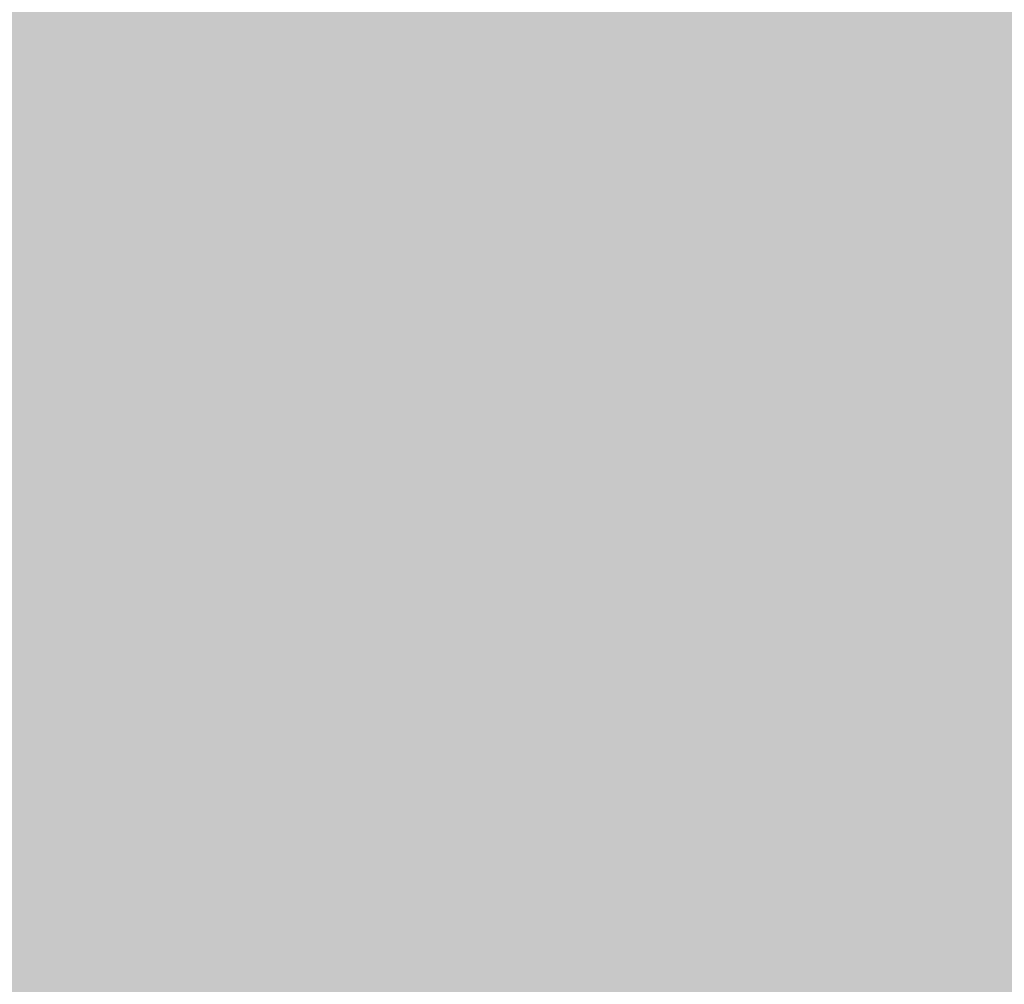
# Model space of a CAD drawing. Units: feet. Extents: x 3168 to 4724, y 827 to 1477.
# Tile 16 of 256: x 3257.5 to 3270.27, y 1074.89 to 1087.4. Entities that reach past the tile are written whole.
import ezdxf

# ---------------------------------------------------------------- set-up
doc = ezdxf.new("R2010")
doc.units = ezdxf.units.FT
doc.layers.add('A-ELEV-PATT', color=8, linetype='Continuous', lineweight=13)

msp = doc.modelspace()

# ---------------------------------------------------------------- hatches: boundary and pattern name
at = {"layer": 'A-ELEV-PATT'}
h = msp.add_hatch(color=256, dxfattribs=at)
h.dxf.hatch_style = 1
edge = h.paths.add_edge_path()
edge.add_ellipse((3552.906, 979.22), major_axis=(36.745, 0), ratio=0.484848, start_angle=0, end_angle=360)
edge = h.paths.add_edge_path()
edge.add_ellipse((3559.892, 929.252), major_axis=(36.745, 0), ratio=0.484848, start_angle=0, end_angle=360)
edge = h.paths.add_edge_path()
edge.add_line((3299.317, 1198.606), (3479.917, 1198.606))
edge.add_line((3479.917, 1198.606), (3479.917, 1209.869))
edge.add_spline(control_points=[(3479.917, 1209.869), (3464.301, 1209.869), (3448.686, 1209.869), (3410.949, 1209.869), (3388.828, 1209.869), (3355.647, 1209.869), (3344.586, 1209.869), (3327.996, 1209.869), (3322.466, 1209.869), (3314.17, 1209.869), (3311.405, 1209.869), (3307.257, 1209.869), (3305.875, 1209.869), (3303.801, 1209.869), (3303.11, 1209.869), (3302.073, 1209.869), (3301.727, 1209.869), (3301.209, 1209.869), (3301.036, 1209.869), (3300.777, 1209.869), (3300.69, 1209.869), (3300.561, 1209.869), (3300.517, 1209.869), (3300.453, 1209.869), (3300.431, 1209.869), (3300.399, 1209.869), (3300.388, 1209.869), (3300.366, 1209.869), (3300.346, 1209.869), (3300.346, 1209.869), (3300.346, 1209.869), (3300.343, 1209.869), (3300.341, 1209.869), (3300.338, 1209.869), (3300.337, 1209.869), (3300.334, 1209.869), (3300.332, 1209.869), (3300.326, 1209.869), (3300.321, 1209.869), (3300.311, 1209.869), (3300.306, 1209.869), (3300.291, 1209.869), (3300.28, 1209.869), (3300.232, 1209.869), (3300.195, 1209.869), (3299.951, 1209.871), (3299.745, 1209.874), (3299.437, 1209.883), (3299.334, 1209.887), (3299.181, 1209.893), (3299.13, 1209.895), (3298.652, 1209.917), (3298.229, 1209.946), (3297.602, 1210.002), (3297.393, 1210.023), (3297.083, 1210.058), (3296.979, 1210.07), (3296.293, 1210.155), (3295.718, 1210.243), (3294.869, 1210.399), (3294.588, 1210.454), (3294.169, 1210.543), (3294.03, 1210.574), (3291.707, 1211.101), (3289.654, 1211.813), (3285.776, 1213.564), (3283.951, 1214.603), (3280.512, 1216.98), (3278.897, 1218.318), (3276.38, 1220.829), (3275.416, 1221.918), (3274.039, 1223.708), (3273.581, 1224.35), (3273.143, 1225.016)], knot_values=[39.119033, 39.119033, 39.119033, 39.119033, 39.286353, 39.286353, 39.523379, 39.523379, 39.641892, 39.641892, 39.701148, 39.701148, 39.730777, 39.730777, 39.745591, 39.745591, 39.752998, 39.752998, 39.756701, 39.756701, 39.758553, 39.758553, 39.759479, 39.759479, 39.759942, 39.759942, 39.760173, 39.760173, 39.760289, 39.760289, 39.760405, 39.760405, 39.760463, 39.760463, 39.763389, 39.763389, 39.764851, 39.764851, 39.767304, 39.767304, 39.773825, 39.773825, 39.78057, 39.78057, 39.79477, 39.79477, 39.845194, 39.845194, 40.126715, 40.126715, 40.267476, 40.267476, 40.337856, 40.337856, 40.927023, 40.927023, 41.221606, 41.221606, 41.368898, 41.368898, 42.202622, 42.202622, 42.619485, 42.619485, 42.827916, 42.827916, 46.118323, 46.118323, 49.408731, 49.408731, 52.699139, 52.699139, 54.927489, 54.927489, 56.104228, 56.104228, 56.104228, 56.104228], weights=[1, 1, 1, 1, 1, 1, 1, 1, 1, 1, 1, 1, 1, 1, 1, 1, 1, 1, 1, 1, 1, 1, 1, 1, 1, 1, 1, 1, 1, 1, 1, 1, 1, 1, 1, 1, 1, 1, 1, 1, 1, 1, 1, 1, 1, 1, 1, 1, 1, 1, 1, 1, 1, 1, 1, 1, 1, 1, 1, 1, 1, 1, 1, 1, 1, 1, 1, 1, 1, 1, 1, 1, 1, 1], degree=3, periodic=0)
edge.add_line((3273.143, 1225.016), (3273.143, 1099.016))
edge.add_line((3273.143, 1099.016), (3299.317, 1099.016))
edge.add_line((3299.317, 1099.016), (3299.317, 1198.606))
edge = h.paths.add_edge_path()
edge.add_line((3304.758, 1324.158), (3479.917, 1324.158))
edge.add_line((3479.917, 1324.158), (3479.917, 1335.715))
edge.add_line((3479.917, 1335.715), (3269.162, 1335.715))
edge.add_spline(control_points=[(3269.162, 1335.715), (3264.024, 1335.715), (3258.364, 1328.958), (3259.264, 1323.9)], knot_values=[0, 0, 0, 0, 15.412191, 15.412191, 15.412191, 15.412191], degree=3, periodic=0)
edge.add_line((3259.264, 1323.9), (3265.517, 1288.769))
edge.add_line((3265.517, 1288.769), (3275.265, 1261.546))
edge.add_line((3275.265, 1261.546), (3304.758, 1261.546))
edge.add_line((3304.758, 1261.546), (3304.758, 1324.158))
h = msp.add_hatch(color=256, dxfattribs=at)
h.dxf.hatch_style = 1
h.paths.add_polyline_path([(3384.525, 1099.016), (3335.029, 1099.016), (3299.317, 1099.016), (3273.143, 1099.016), (3217.565, 1099.016), (3168.069, 827.116), (3335.029, 827.116)])

doc.saveas('drawing.dxf')
